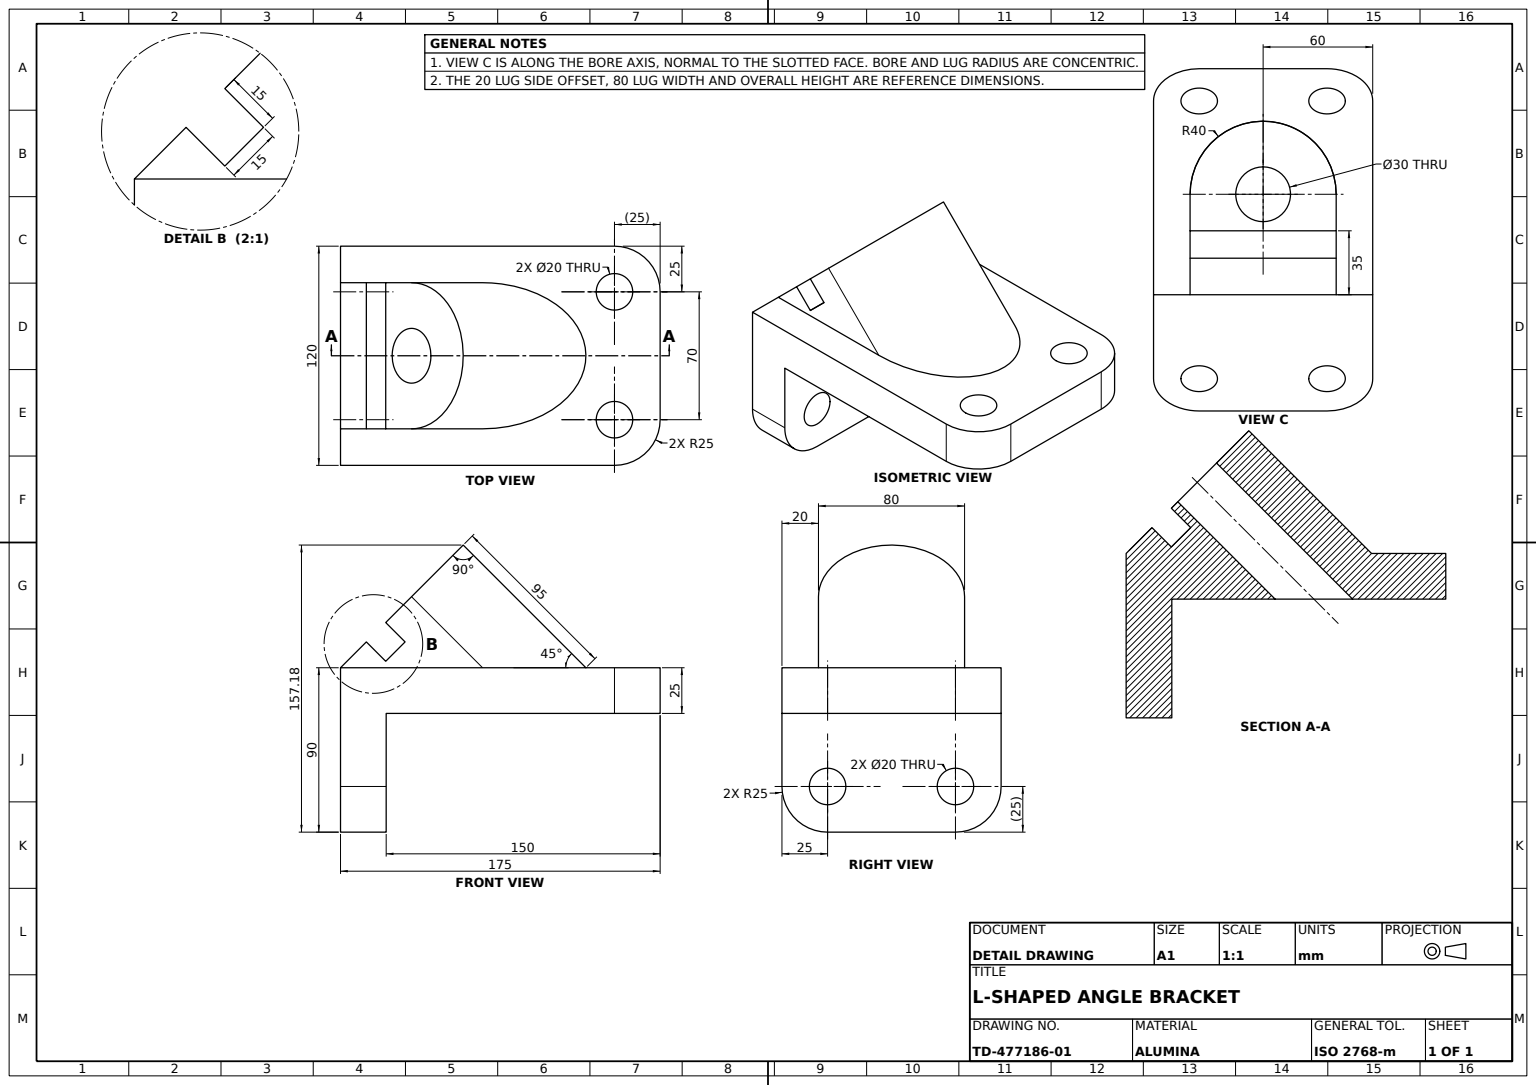
from build123d import *

# Parameters (mm, degrees)
BASE_PLATE_DEPTH            = 25
UPRIGHT_FLANGE_SKETCH_W     = 150
UPRIGHT_FLANGE_SKETCH_H     = 25
UPRIGHT_FLANGE_DEPTH        = 60
BASE_MOUNTING_HOLES_REACH   = 207.73
BASE_HOLES_SKETCH_R         = 10
LUG_SUPPORT_DEPTH           = 60
LUG_CLEARANCE_CUT_REACH     = 207.73
LUG_BORE_30_REACH           = 207.73
LUG_BORE_SKETCH_R           = 15
LUG_SLOT_SKETCH_W           = 80
LUG_SLOT_SKETCH_H           = 15
LUG_SLOT_DEPTH              = 15
FLANGE_CORNER_FILLETS_R25_R = 25
FLANGE_MOUNTING_HOLES_REACH = 207.73
FLANGE_HOLES_SKETCH_R       = 10


with BuildPart() as part:
    # Base Plate Sketch → Base Plate (new body)
    with BuildSketch(Plane.XY):
        with BuildLine():
            Line((-35, -90), (35, -90))
            ThreePointArc((35, -90), (52.67766953, -82.67766953), (60, -65))
            Line((60, -65), (60, 0))
            Line((60, 0), (-60, 0))
            Line((-60, 0), (-60, -65))
            ThreePointArc((-60, -65), (-52.67766953, -82.67766953), (-35, -90))
        make_face()
    extrude(amount=-BASE_PLATE_DEPTH)

    # Upright Flange Sketch → Upright Flange (add, symmetric)
    with BuildSketch(Plane(origin=(0, 0, 0), x_dir=(0, 0, -1), z_dir=(1, 0, 0))):
        with Locations((100, -12.5)):
            Rectangle(UPRIGHT_FLANGE_SKETCH_W, UPRIGHT_FLANGE_SKETCH_H)
    extrude(amount=UPRIGHT_FLANGE_DEPTH, both=True)

    # Base Holes Sketch → Base Mounting Holes (cut, up to next)
    with BuildSketch(Plane.XY, mode=Mode.PRIVATE) as base_mounting_holes_sk1:
        with Locations((35, -65)):
            Circle(BASE_HOLES_SKETCH_R)
    base_mounting_holes_tool1 = extrude(base_mounting_holes_sk1.sketch, amount=-BASE_MOUNTING_HOLES_REACH, mode=Mode.PRIVATE) & part.part
    # Base Holes Sketch → Base Mounting Holes (cut, up to next)
    with BuildSketch(Plane.XY, mode=Mode.PRIVATE) as base_mounting_holes_sk2:
        with Locations((-35, -65)):
            Circle(BASE_HOLES_SKETCH_R)
    base_mounting_holes_tool2 = extrude(base_mounting_holes_sk2.sketch, amount=-BASE_MOUNTING_HOLES_REACH, mode=Mode.PRIVATE) & part.part
    add(base_mounting_holes_tool1.solids().sort_by_distance((35, -65, 0))[0], mode=Mode.SUBTRACT)
    add(base_mounting_holes_tool2.solids().sort_by_distance((-35, -65, 0))[0], mode=Mode.SUBTRACT)

    # Lug Support Sketch → Lug Support (add, symmetric)
    with BuildSketch(Plane(origin=(0, 0, 0), x_dir=(0, 0, -1), z_dir=(1, 0, 0))):
        Polygon((0, 0), (67.175144213, 67.175144213), (134.350288425, 0), align=None)
    extrude(amount=LUG_SUPPORT_DEPTH, both=True)

    # Lug Clearance Cut: up to this face of the body (flat: up to its plane)
    lug_clearance_cut_end = Plane(part.part.faces().sort_by_distance((0, 0, -154.675144213))[0])
    # Lug Clearance Sketch → Lug Clearance Cut (cut, up to the picked face)
    with BuildSketch(Plane(origin=(0, 0, 0), x_dir=(1, 0, 0), z_dir=(0, 0.7071067811865435, 0.7071067811865517)), mode=Mode.PRIVATE) as lug_clearance_cut_sk1:
        with BuildLine():
            Line((40, 55), (40, 0))
            Line((40, 0), (60, 0))
            Line((60, 0), (60, 95))
            Line((60, 95), (-2.46e-07, 95))
            ThreePointArc((-2.46e-07, 95), (28.28427116, 83.284271335), (40, 55))
        make_face()
    lug_clearance_cut_tool1 = split(extrude(lug_clearance_cut_sk1.sketch, amount=-LUG_CLEARANCE_CUT_REACH, mode=Mode.PRIVATE), bisect_by=lug_clearance_cut_end, keep=Keep.BOTH, mode=Mode.PRIVATE)
    # Lug Clearance Sketch → Lug Clearance Cut (cut, up to the picked face)
    with BuildSketch(Plane(origin=(0, 0, 0), x_dir=(1, 0, 0), z_dir=(0, 0.7071067811865435, 0.7071067811865517)), mode=Mode.PRIVATE) as lug_clearance_cut_sk2:
        with BuildLine():
            Line((-60, 0), (-40, 0))
            Line((-40, 0), (-40, 55))
            ThreePointArc((-40, 55), (-28.284271335, 83.28427116), (-2.46e-07, 95))
            Line((-2.46e-07, 95), (-60, 95))
            Line((-60, 95), (-60, 0))
        make_face()
    lug_clearance_cut_tool2 = split(extrude(lug_clearance_cut_sk2.sketch, amount=-LUG_CLEARANCE_CUT_REACH, mode=Mode.PRIVATE), bisect_by=lug_clearance_cut_end, keep=Keep.BOTH, mode=Mode.PRIVATE)
    add(lug_clearance_cut_tool1.solids().sort_by(Axis((47.101904, 37.761408, -37.761408), (0, -0.7071067811865435, -0.7071067811865517)))[0], mode=Mode.SUBTRACT)
    add(lug_clearance_cut_tool2.solids().sort_by(Axis((-47.101904, 37.761408, -37.761408), (0, -0.7071067811865435, -0.7071067811865517)))[0], mode=Mode.SUBTRACT)

    # Lug Bore Ø30: up to this plane
    lug_bore_30_end = Plane(origin=(60, -25, -175), z_dir=(0, 1, 0))
    # Lug Bore Sketch → Lug Bore Ø30 (cut, up to the surface)
    with BuildSketch(Plane(origin=(0, 0, 0), x_dir=(1, 0, 0), z_dir=(0, 0.7071067811865435, 0.7071067811865517)), mode=Mode.PRIVATE) as lug_bore_30_sk1:
        with Locations(Location((0, 55, 0), (0, 0, 270))):
            Circle(LUG_BORE_SKETCH_R)
    lug_bore_30_tool1 = split(extrude(lug_bore_30_sk1.sketch, amount=-LUG_BORE_30_REACH, mode=Mode.PRIVATE), bisect_by=lug_bore_30_end, keep=Keep.BOTH, mode=Mode.PRIVATE)
    add(lug_bore_30_tool1.solids().sort_by_distance((0, 38.890873, -38.890873))[0], mode=Mode.SUBTRACT)

    # Lug Slot Sketch → Lug Slot (cut)
    with BuildSketch(Plane(origin=(0, 0, 0), x_dir=(1, 0, 0), z_dir=(0, 0.7071067811865435, 0.7071067811865517))):
        with Locations((0, 27.5)):
            Rectangle(LUG_SLOT_SKETCH_W, LUG_SLOT_SKETCH_H)
    extrude(amount=-LUG_SLOT_DEPTH, mode=Mode.SUBTRACT)

    # Flange Corner Fillets R25
    flange_corner_fillets_r25_edges = [part.edges().sort_by_distance(p)[0] for p in [
        (-60, -12.5, -175),
        (60, -12.5, -175),
    ]]
    fillet(flange_corner_fillets_r25_edges, radius=FLANGE_CORNER_FILLETS_R25_R)

    # Flange Holes Sketch → Flange Mounting Holes (cut, up to next)
    with BuildSketch(Plane(origin=(0, 0, 0), x_dir=(1, 0, 0), z_dir=(0, 1, 0)), mode=Mode.PRIVATE) as flange_mounting_holes_sk1:
        with Locations(Location((-35, 150, 0), (0, 0, 180))):
            Circle(FLANGE_HOLES_SKETCH_R)
    flange_mounting_holes_tool1 = extrude(flange_mounting_holes_sk1.sketch, amount=-FLANGE_MOUNTING_HOLES_REACH, mode=Mode.PRIVATE) & part.part
    # Flange Holes Sketch → Flange Mounting Holes (cut, up to next)
    with BuildSketch(Plane(origin=(0, 0, 0), x_dir=(1, 0, 0), z_dir=(0, 1, 0)), mode=Mode.PRIVATE) as flange_mounting_holes_sk2:
        with Locations(Location((35, 150, 0), (0, 0, 180))):
            Circle(FLANGE_HOLES_SKETCH_R)
    flange_mounting_holes_tool2 = extrude(flange_mounting_holes_sk2.sketch, amount=-FLANGE_MOUNTING_HOLES_REACH, mode=Mode.PRIVATE) & part.part
    add(flange_mounting_holes_tool1.solids().sort_by_distance((-35, 0, -150))[0], mode=Mode.SUBTRACT)
    add(flange_mounting_holes_tool2.solids().sort_by_distance((35, 0, -150))[0], mode=Mode.SUBTRACT)


solid = part.part
